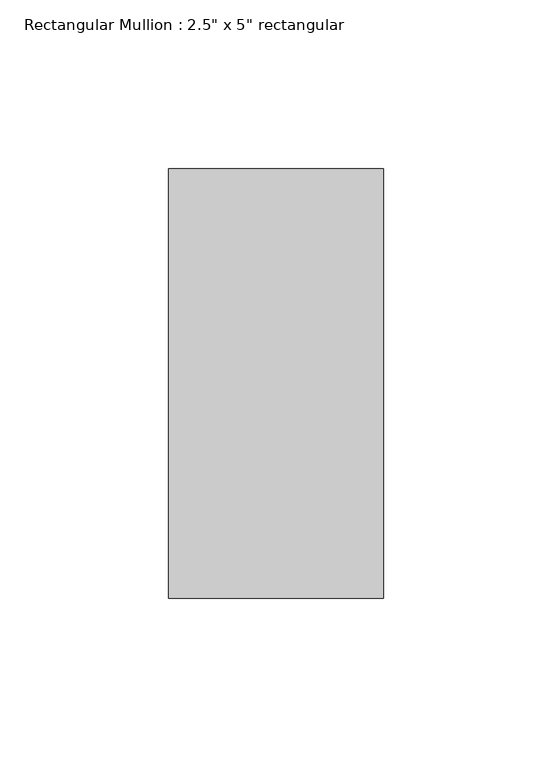
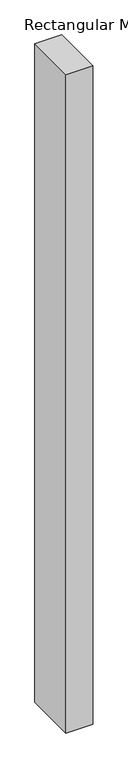
"""IFC4 building model written with IfcOpenShell, lengths in millimetres: member geometry."""

from ifc_helpers import new_model, si_unit, frame, origin, place, context, project, spatial, polyline, outline, extrude, source, transform, mapped, element, save


def member_16047d0f(model_context):
    return source(origin(), model_context, "Body", "SweptSolid", [
        extrude(outline(polyline([(31.75, 63.5), (31.75, -63.5), (-31.75, -63.5), (-31.75, 63.5), (31.75, 63.5)])), frame((0.0, 0.0, -1643.8504197), z_axis=(0.0, 0.0, 1.0), x_axis=(1.0, 0.0, 0.0)), (0.0, 0.0, 1.0), 1643.8504197),
    ])


if __name__ == "__main__":
    model = new_model("IFC4")
    model_context = context("Model", 3, world=origin())
    ifc_project = project(units=[si_unit("LENGTHUNIT", "METRE", prefix="MILLI")], contexts=[model_context])
    site = spatial("IfcSite", under=ifc_project)
    building = spatial("IfcBuilding", under=site)
    placement = place(None, origin())
    member_shape = member_16047d0f(model_context)
    element("IfcMember", 1, ObjectType="Rectangular Mullion : 2.5\" x 5\" rectangular", at=placement, inside=building, context=model_context, shape_type="MappedRepresentation", body=[
        mapped(member_shape, transform((0.0, 0.0, 0.0), x_axis=(1.0, 0.0, 0.0), y_axis=(0.0, 1.0, 0.0), z_axis=(0.0, 0.0, 1.0))),
    ])
    save(model, "model.ifc")

# Revit data of these elements
# Type "Rectangular Mullion : 2.5\" x 5\" rectangular"
#   built-in parameter 1007304 = 0.416667 (stored number, unit not read)
#   built-in parameter 1007301 = 0.104167 (stored number, unit not read)
#   built-in parameter 1007300 = 0.104167 (stored number, unit not read)
# Element 1 (IfcMember, "Rectangular Mullion : 2.5\" x 5\" rectangular")
#   Materials on its faces: "Aluminum"
# Materials
#   "Aluminum": class "Metal", colour RGB 247 247 247, transparency 0, Description = "Aluminum 6061", Cost = 0
